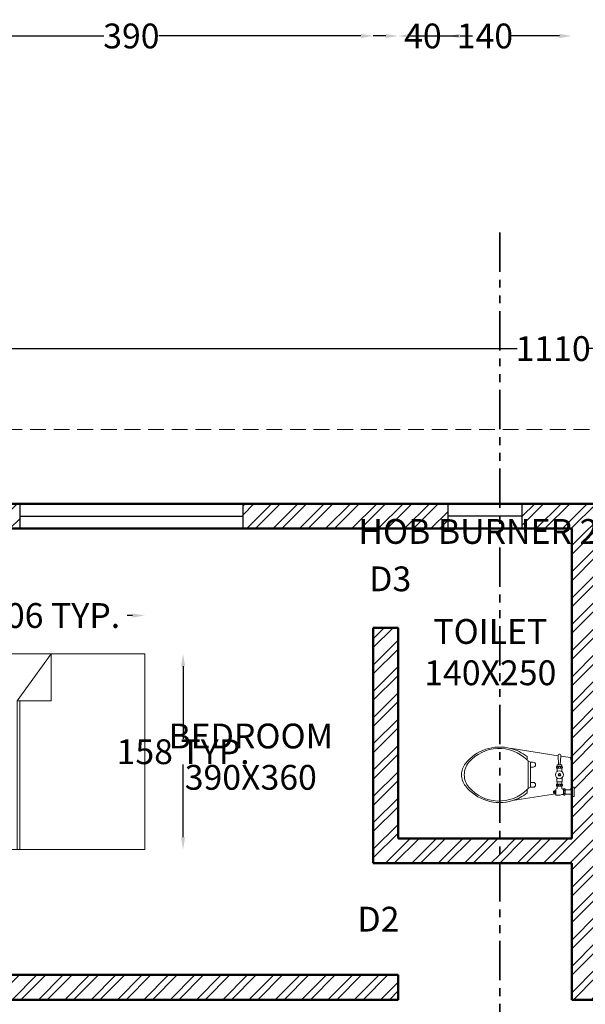
# Model space of a CAD drawing. Units: centimetres. Extents: x 10444 to 13814, y 8288 to 11191.
# Tile 5 of 9: x 10810 to 11266, y 10397 to 11191. Entities that reach past the tile are written whole.
import ezdxf

# ---------------------------------------------------------------- set-up
doc = ezdxf.new("R2010")
doc.units = ezdxf.units.CM
doc.header["$MEASUREMENT"] = 0
doc.linetypes.add('DASHED', pattern=[19.05, 12.7, -6.35])
doc.linetypes.add('PHANTOM', pattern=[63.5, 31.75, -6.35, 6.35, -6.35, 6.35, -6.35])
for name, color, linetype, lineweight in [('A-ANNO-DIMS', 2, 'Continuous', 18), ('A-ANNO-SYMB-SECT', 1, 'PHANTOM', 35), ('A-ANNO-TEXT', 7, 'Continuous', 25), ('A-AREA-IDEN', 3, 'Continuous', 25), ('A-FLOR-FIXT', 9, 'Continuous', 18), ('A-FURN', 8, 'Continuous', 18), ('A-GLAZ', 4, 'Continuous', 25), ('A-ROOF-OVHD', 6, 'DASHED', 18), ('A-WALL', 7, 'Continuous', 50), ('A-WALL-PATT', 8, 'Continuous', 13)]:
    doc.layers.add(name, color=color, linetype=linetype, lineweight=lineweight)
doc.styles.get("Standard").update_dxf_attribs({"font": 'arial.ttf'})
doc.dimstyles.get("Standard").update_dxf_attribs({"dimtxt": 20, "dimasz": 10, "dimexe": 0.18, "dimexo": 0.0625, "dimgap": 0.09, "dimtad": 0, "dimtih": 1, "dimtoh": 1, "dimdec": 0, "dimzin": 0, "dimdsep": 46, "dimtxsty": 'Standard', "dimcen": 0.09, "dimse1": 1, "dimse2": 1, "dimadec": 0, "dimazin": 0, "dimtfac": 1, "dimtdec": 0, "dimtofl": 0, "dimtmove": 0, "dimatfit": 3, "dimfxl": 1, "dimtolj": 1, "dimtzin": 0, "dimarcsym": 0})

# ---------------------------------------------------------------- blocks, each defined once
blk = doc.blocks.new('TOILETY')
for p, q in [((2296.18, 1053.04), (2296.18, 1053.32)), ((2296.61, 1052.51), (2296.98, 1052.51)), ((2296.98, 1052.51), (2297.74, 1052.51)), ((2297.74, 1052.61), (2297.74, 1052.53)), ((2297.74, 1052.53), (2297.74, 1052.51)), ((2297.74, 1052.51), (2297.74, 1050.24)), ((2297.74, 1050.24), (2297.74, 1050.17)), ((2303.23, 1052.05), (2303.23, 1050.7)), ((2307.26, 1052.61), (2307.26, 1052.53)), ((2307.26, 1052.53), (2307.26, 1052.51)), ((2307.26, 1052.51), (2307.26, 1050.24)), ((2307.26, 1050.24), (2307.26, 1050.17)), ((2297.18, 1037.38), (2297.18, 1038.67)), ((2299.5, 1038.67), (2299.5, 1037.38)), ((2306.94, 1038.67), (2306.94, 1037.38)), ((2309.26, 1037.38), (2309.26, 1038.67)), ((2296.53, 1036.19), (2297.18, 1037.38)), ((2299.5, 1037.38), (2297.18, 1037.38)), ((2303.22, 1037.38), (2299.5, 1037.38)), ((2303.22, 1037.38), (2306.94, 1037.38)), ((2306.94, 1037.38), (2309.26, 1037.38)), ((2309.9, 1036.19), (2309.26, 1037.38))]:
    blk.add_line(p, q)
for points in [[(2293.85, 1057.29), (2293.28, 1057.29, -0.293225), (2292.64, 1058.42), (2294.98, 1058.42), (2297.17, 1058.42, -0.293225), (2296.54, 1057.29), (2295.97, 1057.29)], [(2293.85, 1054.1), (2293.63, 1054.1, 0.913215), (2293.63, 1053.32)], [(2294.98, 1057.29), (2293.85, 1057.29, -0.293225)], [(2294.91, 1054.1), (2293.85, 1054.1, 0.913215)], [(2294.91, 1054.1), (2295.97, 1054.1, -0.913215)], [(2294.98, 1057.29), (2295.97, 1057.29, 0.335115)], [(2295.97, 1056.9, -0.066772), (2311.57, 1056.74, -11.173493)], [(2295.97, 1054.1), (2296.18, 1054.1, -0.913215), (2296.18, 1053.32), (2296.11, 1053.32)], [(2312.2, 1051.98), (2311.57, 1056.74, 0.064477)], [(2290.73, 1028.75), (2293.96, 1049.64, -0.075157)], [(2297.78, 1052.66, 0.071269), (2297.81, 1052.53, 0.085783), (2297.9, 1052.35, 0.10607), (2298.04, 1052.23, 0.126822), (2298.2, 1052.19, 0.126822), (2298.36, 1052.23, 0.10607), (2298.5, 1052.35, 0.085783), (2298.59, 1052.53, 0.071269), (2298.62, 1052.66, 0.075445)], [(2297.78, 1050.12, -0.056795), (2297.81, 1050.29, -0.085783), (2297.9, 1050.46, -0.10607), (2298.04, 1050.59, -0.126822), (2298.2, 1050.63, -0.126822), (2298.36, 1050.59, -0.10607), (2298.5, 1050.46, -0.085783), (2298.59, 1050.29, -0.056795), (2298.62, 1050.12, -0.075445)], [(2298.66, 1052.58, 0.236068), (2298.84, 1052.47), (2299.76, 1052.47, 0.868488)], [(2298.66, 1050.17, -0.236068), (2298.84, 1050.28), (2299.76, 1050.28, -0.868488)], [(2306.34, 1052.58, -0.236068), (2306.17, 1052.47), (2304.79, 1052.47, -0.947474)], [(2306.34, 1050.17, 0.236068), (2306.17, 1050.28), (2304.79, 1050.28, 0.947474)], [(2307.23, 1052.66, -0.071269), (2307.19, 1052.53, -0.085783), (2307.1, 1052.35, -0.10607), (2306.96, 1052.23, -0.126822), (2306.8, 1052.19, -0.126822), (2306.65, 1052.23, -0.10607), (2306.5, 1052.35, -0.085783), (2306.41, 1052.53, -0.071269), (2306.38, 1052.66, -0.075445)], [(2307.23, 1050.12, 0.056795), (2307.19, 1050.29, 0.085783), (2307.1, 1050.46, 0.10607), (2306.96, 1050.59, 0.126822), (2306.8, 1050.63, 0.126822), (2306.65, 1050.59, 0.10607), (2306.5, 1050.46, 0.085783), (2306.41, 1050.29, 0.056795), (2306.38, 1050.12, 0.075445)], [(2307.26, 1052.51, 0.414214), (2307.4, 1052.44), (2307.9, 1052.47, -0.274044), (2308.04, 1052.4), (2308.04, 1051.9)], [(2307.26, 1050.24, -0.414214), (2307.4, 1050.31), (2307.9, 1050.28, 0.274044), (2308.04, 1050.35), (2308.04, 1050.84)], [(2308.04, 1051.9, 0.386607), (2308.25, 1051.76), (2312.2, 1051.98, -0.016038)], [(2308.04, 1050.84, -0.386607), (2308.25, 1050.98), (2312.4, 1050.75, 0.016063)], [(2312.2, 1051.98), (2312.68, 1052.01, -0.016603), (2312.71, 1052.01, -1.33807)], [(2312.4, 1050.75), (2312.68, 1050.74, 0.016603), (2312.71, 1050.74, 1.33807)], [(2315.84, 1028.5), (2312.4, 1050.75, 0.07524)], [(2312.71, 1052.01, -0.398884), (2313.25, 1051.55), (2313.25, 1051.37)], [(2312.71, 1050.74, 0.398884), (2313.25, 1051.2), (2313.25, 1051.37)], [(2296.03, 1035.7, 0.434217), (2297.18, 1007.59, 0.182634), (2303.22, 1005.38, 2.693815)], [(2294.42, 1035.7, 0.094048), (2290.73, 1028.75, 0.16845)], [(2296.03, 1035.7), (2294.42, 1035.7, 0.416606)], [(2296.53, 1036.19, 0.008985), (2296.03, 1035.7, 0.182634)], [(2303.22, 1036.19), (2296.53, 1036.19, 0.008985)], [(2303.22, 1036.19), (2309.9, 1036.19, -0.444938)], [(2310.4, 1035.7, -0.434217), (2309.26, 1007.59, -0.182634), (2303.22, 1005.38, -2.693815)], [(2309.9, 1036.19, -0.008985), (2310.4, 1035.7, -0.182634)], [(2310.4, 1035.7), (2312.01, 1035.7, -0.416606)], [(2312.01, 1035.7, -0.105447), (2315.97, 1027.83, -0.16845)], [(2290.73, 1028.75, 0.310397), (2297.82, 1005.91, 0.16845), (2303.22, 1004.04, 2.883082)], [(2315.97, 1027.83, -0.298065), (2308.61, 1005.91, -0.16845), (2303.22, 1004.04, -2.883082)], [(2315.97, 1027.83, 0.006132), (2315.84, 1028.5, 0.069947)]]:
    blk.add_lwpolyline(points, format="xyb")
for points in [[(2293.63, 1053.32), (2293.63, 1052.54), (2293.28, 1051.76), (2293.28, 1049.78)], [(2296.18, 1053.32), (2293.63, 1053.32)], [(2293.85, 1054.1), (2293.85, 1057.29)], [(2295.97, 1056.9), (2295.97, 1057.29)], [(2295.97, 1054.1), (2295.97, 1056.9)], [(2293.96, 1049.64), (2293.35, 1049.64), (2293.28, 1049.78)], [(2294.24, 1049.64), (2293.96, 1049.64)], [(2294.17, 1049.46), (2294.24, 1049.46)], [(2294.34, 1048.89), (2294.17, 1048.89), (2294.17, 1049.46)], [(2294.17, 1049.46), (2294.45, 1049.38), (2294.81, 1049.46), (2295.16, 1049.38), (2295.44, 1049.46)], [(2294.17, 1048.89), (2294.45, 1048.96), (2294.81, 1048.89), (2295.16, 1048.96), (2295.44, 1048.89)], [(2294.24, 1049.46), (2294.24, 1049.64)], [(2295.37, 1049.64), (2294.24, 1049.64)], [(2294.24, 1049.46), (2295.37, 1049.46)], [(2294.34, 1048.89), (2294.34, 1048.51), (2294.58, 1048.51)], [(2295.26, 1048.89), (2294.34, 1048.89)], [(2294.45, 1048.96), (2294.45, 1049.38)], [(2294.58, 1048.51), (2295.26, 1048.51), (2295.26, 1048.89)], [(2295.16, 1048.96), (2295.16, 1049.38)], [(2295.37, 1049.46), (2295.44, 1049.46), (2295.44, 1048.89), (2295.26, 1048.89)], [(2296.32, 1049.78), (2296.25, 1049.64), (2295.37, 1049.64)], [(2295.37, 1049.46), (2295.37, 1049.64)], [(2296.33, 1049.78), (2296.56, 1050.24)], [(2296.56, 1050.24), (2297.74, 1050.24)], [(2298.66, 1050.17), (2298.66, 1052.61)], [(2299.76, 1052.51), (2299.76, 1052.72), (2301.87, 1052.72)], [(2299.76, 1052.51), (2299.76, 1050.28)], [(2299.76, 1050.28), (2299.76, 1050.06), (2301.84, 1050.06)], [(2306.34, 1050.17), (2306.34, 1052.61)], [(2308.04, 1051.9), (2308.04, 1051.37)], [(2308.04, 1050.84), (2308.04, 1051.37)]]:
    blk.add_lwpolyline(points)
for points in [[(2294.91, 1053.32, 0.06206), (2295.16, 1053.35, 0.075298), (2295.36, 1053.43, 0.107049), (2295.5, 1053.57, 0.150029), (2295.55, 1053.71, 0.150029), (2295.5, 1053.85, 0.107049), (2295.36, 1053.99, 0.075298), (2295.16, 1054.07, 0.06206), (2294.91, 1054.1, 0.06206), (2294.65, 1054.07, 0.075298), (2294.46, 1053.99, 0.107049), (2294.31, 1053.85, 0.150029), (2294.27, 1053.71, 0.150029), (2294.31, 1053.57, 0.107049), (2294.46, 1053.43, 0.075298), (2294.65, 1053.35, 0.06206)], [(2298.63, 1051.37, -0.075445), (2298.59, 1051.15, -0.085783), (2298.5, 1050.97, -0.10607), (2298.36, 1050.85, -0.126822), (2298.2, 1050.81, -0.126822), (2298.04, 1050.85, -0.10607), (2297.9, 1050.97, -0.085783), (2297.81, 1051.15, -0.075445), (2297.78, 1051.37, -0.075445), (2297.81, 1051.6, -0.085783), (2297.9, 1051.77, -0.10607), (2298.04, 1051.9, -0.126822), (2298.2, 1051.94, -0.126822), (2298.36, 1051.9, -0.10607), (2298.5, 1051.77, -0.085783), (2298.59, 1051.6, -0.075445)], [(2306.38, 1051.37, 0.075445), (2306.41, 1051.15, 0.085783), (2306.5, 1050.97, 0.10607), (2306.65, 1050.85, 0.126822), (2306.8, 1050.81, 0.126822), (2306.96, 1050.85, 0.10607), (2307.1, 1050.97, 0.085783), (2307.19, 1051.15, 0.075445), (2307.23, 1051.37, 0.075445), (2307.19, 1051.6, 0.085783), (2307.1, 1051.77, 0.10607), (2306.96, 1051.9, 0.126822), (2306.8, 1051.94, 0.126822), (2306.65, 1051.9, 0.10607), (2306.5, 1051.77, 0.085783), (2306.41, 1051.6, 0.075445)]]:
    blk.add_lwpolyline(points, format="xyb", close=True)
blk.add_lwpolyline([(2303.23, 1052.05), (2302.65, 1051.71), (2302.65, 1051.04), (2303.23, 1050.7), (2303.81, 1051.04), (2303.81, 1051.71)], close=True)
blk.add_circle((2303.23, 1051.37), 1.91)
for centre, radius, start, end in [((2293.74, 1053.71), 0.391, 275.1944, 84.8056), ((2296.08, 1053.71), 0.391, 95.1944, 264.8056), ((2296.71, 1053.02), 0.527, 178.4608, 258.8588), ((2298.2, 1052.31), 0.551, 33.3985, 146.6015), ((2306.8, 1052.31), 0.551, 33.3985, 146.6015), ((2298.2, 1050.47), 0.551, 213.3985, 326.6015), ((2306.8, 1050.47), 0.551, 213.3985, 326.6015), ((2298.34, 1038.67), 1.16, 0, 180), ((2308.1, 1038.67), 1.16, 0, 180)]:
    blk.add_arc(centre, radius, start, end)
blk = doc.blocks.new('BED')
for p, q in [((1734.14, 2886.74), (1849.51, 2886.74)), ((1734.14, 2884.74), (1849.51, 2884.74)), ((1849.51, 2886.74), (1886.14, 2860.24)), ((1886.14, 2860.24), (1849.51, 2886.74)), ((1849.51, 2886.74), (1849.51, 2860.24)), ((1849.51, 2860.24), (1886.14, 2860.24))]:
    blk.add_line(p, q)
for points in [[(1734.14, 2787.74), (1886.14, 2787.74), (1886.14, 2985.74), (1734.14, 2985.74)], [(1749.96, 2936.84), (1805.89, 2936.84), (1805.89, 2977.01), (1749.96, 2977.01)], [(1813.22, 2937.77), (1869.15, 2937.77), (1869.15, 2977.94), (1813.22, 2977.94)]]:
    blk.add_lwpolyline(points, close=True)
blk = doc.blocks.new('*D10')
at = {"layer": 'A-ANNO-DIMS', "color": 0, "lineweight": -2, "transparency": 16777216}
for p, q in [((10694.79, 10925.83), (11210.81, 10925.83)), ((11784.79, 10925.83), (11268.77, 10925.83))]:
    blk.add_line(p, q, dxfattribs=at)
at = {"layer": 'A-ANNO-DIMS', "color": 0, "transparency": 16777216}
for points in [[(10694.79, 10927.49), (10694.79, 10924.16), (10684.79, 10925.83)], [(11784.79, 10927.49), (11784.79, 10924.16), (11794.79, 10925.83)]]:
    blk.add_solid(points, dxfattribs=at)
at = {"layer": 'Defpoints', "color": 0, "transparency": 16777216}
for p in [(11794.79, 10925.83), (10684.79, 10800.63), (11794.79, 10800.63)]:
    blk.add_point(p, dxfattribs=at)
at = {"layer": 'A-ANNO-DIMS', "color": 0, "transparency": 16777216, "insert": (11239.79, 10925.83), "char_height": 20, "attachment_point": 5}
blk.add_mtext('\\A1;1110', dxfattribs=at)
blk = doc.blocks.new('WIN-1800')
blk.add_line((0, 10), (180, 10))
blk.add_lwpolyline([(0, 0), (180, 0), (180, 20), (0, 20)], close=True)
blk = doc.blocks.new('WIN-600')
blk.add_line((60, 10), (0, 10))
blk.add_lwpolyline([(0, 0), (60, 0), (60, 20), (0, 20)], close=True)
blk = doc.blocks.new('*D39')
at = {"layer": 'A-ANNO-DIMS', "color": 0, "lineweight": -2, "transparency": 16777216}
for p, q in [((11373.21, 10778.33), (11363.21, 10778.33)), ((11413.21, 10778.33), (11423.21, 10778.33))]:
    blk.add_line(p, q, dxfattribs=at)
at = {"layer": 'A-ANNO-DIMS', "color": 0, "transparency": 16777216}
for points in [[(11373.21, 10780), (11373.21, 10776.66), (11383.21, 10778.33)], [(11413.21, 10780), (11413.21, 10776.66), (11403.21, 10778.33)]]:
    blk.add_solid(points, dxfattribs=at)
at = {"layer": 'Defpoints', "color": 0, "transparency": 16777216}
for p in [(11383.21, 10778.33), (11383.21, 10775.33), (11403.21, 10775.33)]:
    blk.add_point(p, dxfattribs=at)
at = {"layer": 'A-ANNO-DIMS', "color": 0, "transparency": 16777216, "insert": (11217.96, 10778.33), "char_height": 20, "attachment_point": 5}
blk.add_mtext('\\A1;HOB BURNER 20 TYP.', dxfattribs=at)
blk = doc.blocks.new('*D41')
at = {"layer": 'A-ANNO-DIMS', "color": 0, "lineweight": -2, "transparency": 16777216}
for p, q in [((10714.79, 10710.51), (10719, 10710.51)), ((10900.6, 10710.51), (10896.39, 10710.51))]:
    blk.add_line(p, q, dxfattribs=at)
at = {"layer": 'A-ANNO-DIMS', "color": 0, "transparency": 16777216}
for points in [[(10714.79, 10712.17), (10714.79, 10708.84), (10704.79, 10710.51)], [(10900.6, 10712.17), (10900.6, 10708.84), (10910.6, 10710.51)]]:
    blk.add_solid(points, dxfattribs=at)
at = {"layer": 'Defpoints', "color": 0, "transparency": 16777216}
for p in [(10704.79, 10710.51), (10704.79, 10679.63), (10910.6, 10679.63)]:
    blk.add_point(p, dxfattribs=at)
at = {"layer": 'A-ANNO-DIMS', "color": 0, "transparency": 16777216, "insert": (10807.7, 10710.51), "char_height": 20, "attachment_point": 5}
blk.add_mtext('\\A1;BED 206 TYP.', dxfattribs=at)
blk = doc.blocks.new('*D42')
at = {"layer": 'A-ANNO-DIMS', "color": 0, "lineweight": -2, "transparency": 16777216}
for p, q in [((10941.48, 10669.63), (10941.48, 10610.94)), ((10941.48, 10531.63), (10941.48, 10590.33))]:
    blk.add_line(p, q, dxfattribs=at)
at = {"layer": 'A-ANNO-DIMS', "color": 0, "transparency": 16777216}
for points in [[(10939.81, 10669.63), (10943.14, 10669.63), (10941.48, 10679.63)], [(10939.81, 10531.63), (10943.14, 10531.63), (10941.48, 10521.63)]]:
    blk.add_solid(points, dxfattribs=at)
at = {"layer": 'Defpoints', "color": 0, "transparency": 16777216}
for p in [(10910.6, 10679.63), (10941.48, 10679.63), (10910.6, 10521.63)]:
    blk.add_point(p, dxfattribs=at)
at = {"layer": 'A-ANNO-DIMS', "color": 0, "transparency": 16777216, "insert": (10941.48, 10600.63), "char_height": 20, "attachment_point": 5}
blk.add_mtext('\\A1;158 TYP.', dxfattribs=at)
blk = doc.blocks.new('*D53')
at = {"layer": 'A-ANNO-DIMS', "color": 0, "lineweight": -2, "transparency": 16777216}
for p, q in [((11104.79, 11178), (11094.79, 11178)), ((11164.79, 11178), (11174.79, 11178))]:
    blk.add_line(p, q, dxfattribs=at)
at = {"layer": 'A-ANNO-DIMS', "color": 0, "transparency": 16777216}
for points in [[(11104.79, 11179.67), (11104.79, 11176.33), (11114.79, 11178)], [(11164.79, 11179.67), (11164.79, 11176.33), (11154.79, 11178)]]:
    blk.add_solid(points, dxfattribs=at)
at = {"layer": 'Defpoints', "color": 0, "transparency": 16777216}
for p in [(11154.79, 11178), (11154.79, 10800.63), (11114.79, 10780.63)]:
    blk.add_point(p, dxfattribs=at)
at = {"layer": 'A-ANNO-DIMS', "color": 0, "transparency": 16777216, "insert": (11134.79, 11178), "char_height": 20, "attachment_point": 5}
blk.add_mtext('\\A1;40', dxfattribs=at)
blk = doc.blocks.new('*D68')
at = {"layer": 'A-ANNO-DIMS', "color": 0, "lineweight": -2, "transparency": 16777216}
for p, q in [((10714.79, 11178), (10877.64, 11178)), ((11084.79, 11178), (10921.93, 11178))]:
    blk.add_line(p, q, dxfattribs=at)
at = {"layer": 'A-ANNO-DIMS', "color": 0, "transparency": 16777216}
for points in [[(10714.79, 11179.67), (10714.79, 11176.33), (10704.79, 11178)], [(11084.79, 11179.67), (11084.79, 11176.33), (11094.79, 11178)]]:
    blk.add_solid(points, dxfattribs=at)
at = {"layer": 'Defpoints', "color": 0, "transparency": 16777216}
for p in [(11094.79, 11178), (10704.79, 10780.63), (11094.79, 10700.63)]:
    blk.add_point(p, dxfattribs=at)
at = {"layer": 'A-ANNO-DIMS', "color": 0, "transparency": 16777216, "insert": (10899.79, 11178), "char_height": 20, "attachment_point": 5}
blk.add_mtext('\\A1;390', dxfattribs=at)
blk = doc.blocks.new('*D69')
at = {"layer": 'A-ANNO-DIMS', "color": 0, "lineweight": -2, "transparency": 16777216}
for p, q in [((11124.79, 11178), (11163.58, 11178)), ((11244.79, 11178), (11206, 11178))]:
    blk.add_line(p, q, dxfattribs=at)
at = {"layer": 'A-ANNO-DIMS', "color": 0, "transparency": 16777216}
for points in [[(11124.79, 11179.67), (11124.79, 11176.33), (11114.79, 11178)], [(11244.79, 11179.67), (11244.79, 11176.33), (11254.79, 11178)]]:
    blk.add_solid(points, dxfattribs=at)
at = {"layer": 'Defpoints', "color": 0, "transparency": 16777216}
for p in [(11254.79, 11178), (11254.79, 10780.63), (11114.79, 10700.63)]:
    blk.add_point(p, dxfattribs=at)
at = {"layer": 'A-ANNO-DIMS', "color": 0, "transparency": 16777216, "insert": (11184.79, 11178), "char_height": 20, "attachment_point": 5}
blk.add_mtext('\\A1;140', dxfattribs=at)
blk = doc.blocks.new('*D71')
at = {"layer": 'A-ANNO-DIMS', "color": 0, "lineweight": -2, "transparency": 16777216}
for p, q in [((10466.29, 10770.63), (10466.29, 10735.94)), ((10466.29, 10680.63), (10466.29, 10715.33))]:
    blk.add_line(p, q, dxfattribs=at)
at = {"layer": 'A-ANNO-DIMS', "color": 0, "transparency": 16777216}
for points in [[(10464.62, 10770.63), (10467.95, 10770.63), (10466.29, 10780.63)], [(10464.62, 10680.63), (10467.95, 10680.63), (10466.29, 10670.63)]]:
    blk.add_solid(points, dxfattribs=at)
at = {"layer": 'Defpoints', "color": 0, "transparency": 16777216}
for p in [(11594.79, 10780.63), (10466.29, 10670.63), (11674.79, 10670.63)]:
    blk.add_point(p, dxfattribs=at)
at = {"layer": 'A-ANNO-DIMS', "color": 0, "transparency": 16777216, "insert": (10466.29, 10725.63), "char_height": 20, "attachment_point": 5}
blk.add_mtext('\\A1;110', dxfattribs=at)
blk = doc.blocks.new('*D73')
at = {"layer": 'A-ANNO-DIMS', "color": 0, "lineweight": -2, "transparency": 16777216}
for p, q in [((11124.79, 11178), (11163.58, 11178)), ((11244.79, 11178), (11206, 11178))]:
    blk.add_line(p, q, dxfattribs=at)
at = {"layer": 'A-ANNO-DIMS', "color": 0, "transparency": 16777216}
for points in [[(11124.79, 11179.67), (11124.79, 11176.33), (11114.79, 11178)], [(11244.79, 11179.67), (11244.79, 11176.33), (11254.79, 11178)]]:
    blk.add_solid(points, dxfattribs=at)
at = {"layer": 'Defpoints', "color": 0, "transparency": 16777216}
for p in [(11254.79, 11178), (11114.79, 10400.63), (11254.79, 10400.63)]:
    blk.add_point(p, dxfattribs=at)
at = {"layer": 'A-ANNO-DIMS', "color": 0, "transparency": 16777216, "insert": (11184.79, 11178), "char_height": 20, "attachment_point": 5}
blk.add_mtext('\\A1;140', dxfattribs=at)
blk = doc.blocks.new('*D75')
at = {"layer": 'A-ANNO-DIMS', "color": 0, "lineweight": -2, "transparency": 16777216}
for p, q in [((10466.29, 10500.63), (10466.29, 10475.94)), ((10466.29, 10430.63), (10466.29, 10455.33))]:
    blk.add_line(p, q, dxfattribs=at)
at = {"layer": 'A-ANNO-DIMS', "color": 0, "transparency": 16777216}
for points in [[(10464.62, 10500.63), (10467.95, 10500.63), (10466.29, 10510.63)], [(10464.62, 10430.63), (10467.95, 10430.63), (10466.29, 10420.63)]]:
    blk.add_solid(points, dxfattribs=at)
at = {"layer": 'Defpoints', "color": 0, "transparency": 16777216}
for p in [(10466.29, 10510.63), (11784.79, 10510.63), (11794.79, 10420.63)]:
    blk.add_point(p, dxfattribs=at)
at = {"layer": 'A-ANNO-DIMS', "color": 0, "transparency": 16777216, "insert": (10466.29, 10465.63), "char_height": 20, "attachment_point": 5}
blk.add_mtext('\\A1;90', dxfattribs=at)
blk = doc.blocks.new('*D76')
at = {"layer": 'A-ANNO-DIMS', "color": 0, "lineweight": -2, "transparency": 16777216}
for p, q in [((10466.29, 10390.63), (10466.29, 10360.94)), ((10466.29, 10310.63), (10466.29, 10340.33))]:
    blk.add_line(p, q, dxfattribs=at)
at = {"layer": 'A-ANNO-DIMS', "color": 0, "transparency": 16777216}
for points in [[(10464.62, 10390.63), (10467.95, 10390.63), (10466.29, 10400.63)], [(10464.62, 10310.63), (10467.95, 10310.63), (10466.29, 10300.63)]]:
    blk.add_solid(points, dxfattribs=at)
at = {"layer": 'Defpoints', "color": 0, "transparency": 16777216}
for p in [(10466.29, 10400.63), (11114.79, 10400.63), (11054.79, 10300.63)]:
    blk.add_point(p, dxfattribs=at)
at = {"layer": 'A-ANNO-DIMS', "color": 0, "transparency": 16777216, "insert": (10466.29, 10350.63), "char_height": 20, "attachment_point": 5}
blk.add_mtext('\\A1;100', dxfattribs=at)

msp = doc.modelspace()

# ---------------------------------------------------------------- hatches: boundary and pattern name
at = {"layer": 'A-WALL-PATT'}
h = msp.add_hatch(dxfattribs=at)
h.set_pattern_fill('ANSI32', color=256, scale=40)
h.paths.add_polyline_path([(10809.7881, 10800.6336), (10684.7881, 10800.6336), (10684.7881, 10690.6336), (10704.7881, 10690.6336), (10704.7881, 10726.41), (10704.7881, 10780.6336), (10809.7881, 10780.6336)])
h.paths.add_polyline_path([(11154.7881, 10800.6336), (10989.7881, 10800.6336), (10989.7881, 10780.6336), (11114.7881, 10780.6336), (11154.7881, 10780.6336)])
h.paths.add_polyline_path([(11354.7881, 10800.6336), (11214.7881, 10800.6336), (11214.7881, 10780.6336), (11254.7881, 10780.6336), (11254.7881, 10582.9925, -0.00499308), (11254.7881, 10581.0383), (11254.7881, 10571.0719, -0.26947312), (11256.5873, 10571.9821), (11256.5873, 10568.3227), (11256.5873, 10564.4272, -0.26947312), (11254.7881, 10565.3375), (11254.7881, 10530.6336), (11196.6819, 10530.6336), (11196.6819, 10510.6336), (11254.7881, 10510.6336), (11254.7881, 10400.6336), (11274.7881, 10400.6336), (11274.7881, 10420.6336), (11274.7881, 10780.6336), (11354.7881, 10780.6336)])
h.paths.add_polyline_path([(10704.7881, 10510.6336), (10684.7881, 10510.6336), (10684.7881, 10400.6336), (10734.7881, 10400.6336), (10734.7881, 10340.6336), (10754.7881, 10340.6336), (10754.7881, 10400.6336), (11114.7881, 10400.6336), (11114.7881, 10420.6336), (10704.7881, 10420.6336)])
h.paths.add_polyline_path([(11794.7881, 10420.6336), (11364.7881, 10420.6336), (11364.7881, 10400.6336), (11644.7881, 10400.6336), (11644.7881, 10260.6336), (11664.7881, 10260.6336), (11664.7881, 10400.6336), (11794.7881, 10400.6336)])
h.paths.add_polyline_path([(11594.7881, 10670.6336), (11594.7881, 10708.9482, -0.26828041), (11592.9938, 10708.0455), (11592.9938, 10711.9409), (11592.9938, 10715.6003, -0.26828041), (11594.7881, 10714.6976), (11594.7881, 10780.6336), (11654.7881, 10780.6336), (11654.7881, 10800.6336), (11494.7881, 10800.6336), (11494.7881, 10780.6336), (11574.7881, 10780.6336), (11574.7881, 10510.6336), (11594.7881, 10510.6336)])
h.paths.add_polyline_path([(11794.7881, 10800.6336), (11714.7881, 10800.6336), (11714.7881, 10780.6336), (11774.7881, 10780.6336), (11774.7881, 10750.6336), (11794.7881, 10750.6336)])
h.paths.add_polyline_path([(11794.7881, 10670.6336), (11674.7881, 10670.6336), (11674.7881, 10650.6336), (11794.7881, 10650.6336)])
h.paths.add_polyline_path([(11664.7881, 10080.6336), (11644.7881, 10080.6336), (11644.7881, 9940.6336), (11549.7881, 9940.6336), (11549.7881, 9920.6336), (11664.7881, 9920.6336)])
h.paths.add_polyline_path([(11369.7881, 9940.6336), (11274.7881, 9940.6336), (11274.7881, 10300.6336), (11254.7881, 10300.6336), (11254.7881, 9940.6336), (11234.7881, 9940.6336), (11234.7881, 9920.6336), (11369.7881, 9920.6336)])
h.paths.add_polyline_path([(11094.7881, 9940.6336), (11074.7881, 9940.6336), (11074.7881, 10300.6336), (11054.7881, 10300.6336), (11054.7881, 10080.6336), (11054.7881, 9920.6336), (11094.7881, 9920.6336)])
h.paths.add_polyline_path([(11134.7881, 9940.6336), (11114.7881, 9940.6336), (11114.7881, 9920.6336), (11134.7881, 9920.6336)])
h.paths.add_polyline_path([(11174.7881, 9940.6336), (11154.7881, 9940.6336), (11154.7881, 9920.6336), (11174.7881, 9920.6336)])
h.paths.add_polyline_path([(11214.7881, 9940.6336), (11196.6819, 9940.6336), (11196.6819, 9920.6336), (11214.7881, 9920.6336)])
h.paths.add_polyline_path([(10954.7881, 10100.6336), (10874.7881, 10100.6336), (10874.7881, 10080.6336), (10954.7881, 10080.6336)])
h.paths.add_polyline_path([(10814.7881, 10100.6336), (10754.7881, 10100.6336), (10754.7881, 10160.6336), (10734.7881, 10160.6336), (10734.7881, 10080.6336), (10814.7881, 10080.6336)])
h.paths.add_polyline_path([(11255.1494, 10331.8339), (11286.882, 10331.8339), (11286.882, 10373.0481), (11255.1494, 10373.0481)], flags=9)
h.paths.add_polyline_path([(11607.8445, 10630.7128), (11653.5607, 10630.7128), (11653.5607, 10671.927), (11607.8445, 10671.927)], flags=25)
h.paths.add_polyline_path([(11746.8445, 10447.0791), (11792.5607, 10447.0791), (11792.5607, 10488.2933), (11746.8445, 10488.2933)], flags=9)
h.paths.add_polyline_path([(11296.8445, 10388.5791), (11342.5607, 10388.5791), (11342.5607, 10429.7933), (11296.8445, 10429.7933)], flags=9)
h.paths.add_polyline_path([(11376.6416, 10156.0222), (11521.6757, 10156.0222), (11521.6757, 10230.6515), (11376.6416, 10230.6515)], flags=9)
h.paths.add_polyline_path([(11437.3982, 10313.4478), (11545.1881, 10313.4478), (11545.1881, 10354.662), (11437.3982, 10354.662)], flags=25)
h.paths.add_polyline_path([(11655.4027, 10682.0329), (11777.2718, 10682.0329), (11777.2718, 10756.6623), (11655.4027, 10756.6623)], flags=9)
h.paths.add_polyline_path([(11636.2626, 10500.0811), (11758.1316, 10500.0811), (11758.1316, 10574.7105), (11636.2626, 10574.7105)], flags=9)
h.paths.add_polyline_path([(11336.6251, 10562.3234), (11469.2581, 10562.3234), (11469.2581, 10636.9528), (11336.6251, 10636.9528)], flags=9)
h = msp.add_hatch(dxfattribs=at)
h.set_pattern_fill('ANSI32', color=256, scale=40)
h.paths.add_polyline_path([(12933.1062, 10800.6336), (12768.1062, 10800.6336), (12768.1062, 10780.6336), (12933.1062, 10780.6336)])
h.paths.add_polyline_path([(12588.1062, 10800.6336), (12463.1062, 10800.6336), (12463.1062, 10780.6336), (12588.1062, 10780.6336)])
h.paths.add_polyline_path([(12483.1062, 10726.41), (12483.1062, 10780.6336), (12463.1062, 10780.6336), (12463.1062, 10690.6336), (12483.1062, 10690.6336)])
h.paths.add_polyline_path([(12483.1062, 10510.6336), (12463.1062, 10510.6336), (12463.1062, 10400.6336), (12510.094, 10400.6336), (12529.0899, 10420.6336), (12483.1062, 10420.6336)])
h.paths.add_polyline_path([(12699.6814, 10420.6336), (12529.0899, 10420.6336), (12510.094, 10400.6336), (12513.1062, 10400.6336), (12513.1062, 10340.6336), (12533.1062, 10340.6336), (12533.1062, 10400.6336), (12699.64, 10400.6336)])
h.paths.add_polyline_path([(12893.1062, 10420.6336), (12699.6814, 10420.6336), (12699.64, 10400.6336), (12893.1062, 10400.6336)])
h.paths.add_polyline_path([(13129.7438, 10800.6336), (12993.1062, 10800.6336), (12993.1062, 10780.6336), (13033.1062, 10780.6336), (13033.1062, 10600.6336), (13053.1062, 10600.6336), (13053.1062, 10780.6336), (13129.7438, 10780.6336)])
h.paths.add_polyline_path([(13433.1062, 10800.6336), (13309.7438, 10800.6336), (13309.7438, 10780.6336), (13345.5201, 10780.6336), (13353.1062, 10780.6336), (13353.1062, 10600.6336), (13373.1062, 10600.6336), (13373.1062, 10780.6336), (13433.1062, 10780.6336)])
h.paths.add_polyline_path([(13573.1062, 10800.6336), (13493.1062, 10800.6336), (13493.1062, 10780.6336), (13553.1062, 10780.6336), (13553.1062, 10600.6336), (13573.1062, 10600.6336)])
h.paths.add_polyline_path([(13573.1062, 10600.6336), (13553.1062, 10600.6336), (13553.1062, 10420.6336), (13053.1062, 10420.6336), (13053.1062, 10400.6336), (13573.1062, 10400.6336)])
h.paths.add_polyline_path([(13053.1062, 10300.6336), (13033.1062, 10300.6336), (13033.1062, 9940.6336), (13013.1062, 9940.6336), (13013.1062, 9920.6336), (13053.1062, 9920.6336)])
h.paths.add_polyline_path([(12993.1062, 9940.6336), (12975, 9940.6336), (12975, 9920.6336), (12993.1062, 9920.6336)])
h.paths.add_polyline_path([(12953.1062, 9940.6336), (12933.1062, 9940.6336), (12933.1062, 9920.6336), (12953.1062, 9920.6336)])
h.paths.add_polyline_path([(12913.1062, 9940.6336), (12893.1062, 9940.6336), (12893.1062, 9920.6336), (12913.1062, 9920.6336)])
h.paths.add_polyline_path([(12873.1062, 9940.6336), (12853.1062, 9940.6336), (12853.1062, 10300.6336), (12833.1062, 10300.6336), (12833.1062, 9920.6336), (12873.1062, 9920.6336)])
h.paths.add_polyline_path([(12733.1062, 10100.6336), (12699.0201, 10100.6336), (12698.9788, 10080.6336), (12733.1062, 10080.6336)])
h.paths.add_polyline_path([(12699.0201, 10100.6336), (12653.1062, 10100.6336), (12653.1062, 10080.6336), (12698.9788, 10080.6336)])
h.paths.add_polyline_path([(12593.1062, 10100.6336), (12533.1062, 10100.6336), (12533.1062, 10160.6336), (12513.1062, 10160.6336), (12513.1062, 10080.6336), (12593.1062, 10080.6336)])
h.paths.add_polyline_path([(13053.1062, 10600.6336), (13033.1062, 10600.6336), (13033.1062, 10576.2537, -0.00499308), (13033.1062, 10574.2995), (13033.1062, 10564.3331, -0.26947312), (13034.9053, 10565.2433), (13034.9053, 10561.5839), (13034.9053, 10557.6884, -0.26947312), (13033.1062, 10558.5987), (13033.1062, 10530.6336), (12975, 10530.6336), (12975, 10510.6336), (13053.1062, 10510.6336)])
h.paths.add_polyline_path([(12975, 10530.6336), (12893.1062, 10530.6336), (12893.1062, 10600.6336), (12873.1062, 10600.6336), (12873.1062, 10510.6336), (12975, 10510.6336)])
h.paths.add_polyline_path([(12893.1062, 10700.6336), (12873.1062, 10700.6336), (12873.1062, 10600.6336), (12893.1062, 10600.6336)])
h.paths.add_polyline_path([(13373.1062, 10600.6336), (13353.1062, 10600.6336), (13353.1062, 10507.9506), (13373.1062, 10507.9506)], flags=17)
h.paths.add_polyline_path([(13553.1062, 10620.6336), (13453.1062, 10620.6336), (13453.1062, 10600.6336), (13553.1062, 10600.6336)])
h.paths.add_polyline_path([(11114.7881, 10700.6336), (11094.7881, 10700.6336), (11094.7881, 10510.6336), (11196.6819, 10510.6336), (11196.6819, 10530.6336), (11114.7881, 10530.6336)])

# ---------------------------------------------------------------- linework, layer by layer
at = {"layer": 'A-ANNO-SYMB-SECT'}
msp.add_line((11196.6819, 11019.5), (11196.6819, 9676.5), dxfattribs=at)
at = {"layer": 'A-ROOF-OVHD'}
msp.add_line((10684.7881, 10860.6336), (11854.7881, 10860.6336), dxfattribs=at)
at = {"layer": 'A-WALL'}
for p, q in [((10684.7881, 10800.6336), (11794.7881, 10800.6336)), ((10704.7881, 10780.6336), (11114.7881, 10780.6336)), ((11114.7881, 10780.6336), (11254.7881, 10780.6336)), ((11254.7881, 10780.6336), (11254.7881, 10530.6336)), ((11094.7881, 10700.6336), (11094.7881, 10510.6336)), ((11094.7881, 10700.6336), (11114.7881, 10700.6336)), ((11114.7881, 10700.6336), (11114.7881, 10530.6336)), ((11114.7881, 10530.6336), (11254.7881, 10530.6336)), ((11094.7881, 10510.6336), (11254.7881, 10510.6336)), ((11254.7881, 10510.6336), (11254.7881, 10400.6336)), ((10704.7881, 10420.6336), (11114.7881, 10420.6336)), ((11114.7881, 10420.6336), (11114.7881, 10400.6336)), ((11254.7881, 10420.6336), (11254.7881, 10400.6336)), ((10754.7881, 10400.6336), (11114.7881, 10400.6336)), ((11254.7881, 10400.6336), (11274.7881, 10400.6336))]:
    msp.add_line(p, q, dxfattribs=at)
msp.add_lwpolyline([(10734.7881, 9920.6336), (11664.7881, 9920.6336), (11664.7881, 10400.6336), (11794.7881, 10400.6336), (11794.7881, 10800.6336), (10684.7881, 10800.6336), (10684.7881, 10400.6336), (10734.7881, 10400.6336), (10734.7881, 9920.6336)], dxfattribs=at)

# ---------------------------------------------------------------- block references
at = {"layer": 'A-FLOR-FIXT', "xscale": -1.667297040358401, "yscale": 1.667297040358401, "zscale": 1.667297040358401, "rotation": 270}
msp.add_blockref('TOILETY', (9491.8892, 6741.9104), dxfattribs=at)
at = {"layer": 'A-FURN', "xscale": 1.039473684210526, "yscale": 1.039473684210526, "zscale": 1.039473684210526, "rotation": 89.99999999999999}
msp.add_blockref('BED', (13808.3851, 8719.0411), dxfattribs=at)
at = {"layer": 'A-GLAZ'}
for name, p in [('WIN-1800', (10809.788, 10780.634)), ('WIN-600', (11154.788, 10780.634))]:
    msp.add_blockref(name, p, dxfattribs=at)

# ---------------------------------------------------------------- texts
at = {"layer": 'A-ANNO-TEXT', "char_height": 20, "attachment_point": 1}
for s, insert in [('D3', (11091.5, 10750.0819)), ('D2', (11082, 10475.5819))]:
    msp.add_mtext_dynamic_manual_height_columns(s, width=668.5, gutter_width=1, heights=[0], dxfattribs=dict(at, insert=insert))
at = {"layer": 'A-AREA-IDEN', "char_height": 20, "attachment_point": 1}
for s, insert in [('\\pxqc;TOILET\\P140X250', (11114.7881, 10707.6405)), ('\\pxqc;BEDROOM\\P390X360', (10921.7352, 10623.315))]:
    msp.add_mtext_dynamic_manual_height_columns(s, width=148.64167, gutter_width=1, heights=[0], dxfattribs=dict(at, insert=insert))

# ---------------------------------------------------------------- dimensions: what is measured, and where the dimension line sits
at = {"layer": 'A-ANNO-DIMS'}
for base, p1, p2, picture, middle in [((11094.7881, 11178), (10704.7881, 10780.6336), (11094.7881, 10700.6336), '*D68', (10899.7881, 11178)), ((11154.7881, 11178), (11114.7881, 10780.6336), (11154.7881, 10800.6336), '*D53', (11134.7881, 11178)), ((11254.7881, 11178), (11114.7881, 10700.6336), (11254.7881, 10780.6336), '*D69', (11184.7881, 11178)), ((11254.7881, 11178), (11114.7881, 10400.6336), (11254.7881, 10400.6336), '*D73', (11184.7881, 11178))]:
    dim = msp.add_linear_dim(base=base, p1=p1, p2=p2, dimstyle='Standard', override={"dimdec": 0, "dimlfac": 1, "dimrnd": 0, "dimzin": 0, "dimdsep": 46, "dimlunit": 2}, dxfattribs=at)
    dim.commit()
    dim.dimension.update_dxf_attribs({"geometry": picture, "text_midpoint": middle})
dim = msp.add_aligned_dim(p1=(10684.7881, 10800.6336), p2=(11794.7881, 10800.6336), distance=125.1941, dimstyle='Standard', override={"dimclrd": 0, "dimclre": 0, "dimclrt": 0}, dxfattribs=at)
dim.commit()
dim.dimension.update_dxf_attribs({"geometry": '*D10', "text_midpoint": (11239.7881, 10925.8277)})
for base, p1, p2, angle, text, picture, middle in [((11383.2099, 10778.3306), (11403.2099, 10775.3306), (11383.2099, 10775.3306), 180, 'HOB BURNER <> TYP.', '*D39', (11217.9562, 10778.3306)), ((10704.7881, 10710.506), (10910.6039, 10679.6336), (10704.7881, 10679.6336), 180, 'BED <> TYP.', '*D41', (10807.696, 10710.506)), ((10941.4763, 10679.6336), (10910.6039, 10521.6336), (10910.6039, 10679.6336), 90, '<> TYP.', '*D42', (10941.4763, 10600.6336))]:
    dim = msp.add_linear_dim(base=base, p1=p1, p2=p2, angle=angle, text=text, dimstyle='Standard', override={"dimdec": 0, "dimrnd": 0, "dimzin": 0, "dimlunit": 2}, dxfattribs=at)
    dim.commit()
    dim.dimension.update_dxf_attribs({"geometry": picture, "text_midpoint": middle})
for base, p1, p2, picture, middle in [((10466.2881, 10670.6336), (11594.7881, 10780.6336), (11674.7881, 10670.6336), '*D71', (10466.2881, 10725.6336)), ((10466.2881, 10510.6336), (11794.7881, 10420.6336), (11784.7881, 10510.6336), '*D75', (10466.2881, 10465.6336)), ((10466.2881, 10400.6336), (11054.7881, 10300.6336), (11114.7881, 10400.6336), '*D76', (10466.2881, 10350.6336))]:
    dim = msp.add_linear_dim(base=base, p1=p1, p2=p2, angle=90, dimstyle='Standard', override={"dimdec": 0, "dimlfac": 1, "dimrnd": 0, "dimzin": 0, "dimdsep": 46, "dimlunit": 2}, dxfattribs=at)
    dim.commit()
    dim.dimension.update_dxf_attribs({"geometry": picture, "text_midpoint": middle})

doc.saveas('drawing.dxf')
